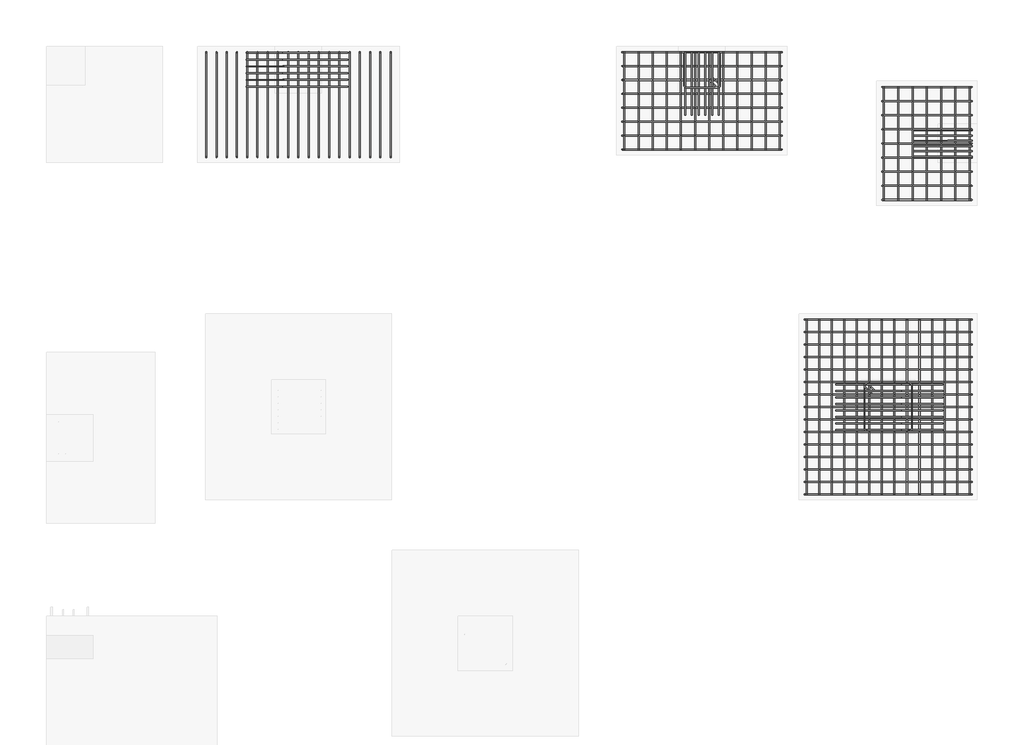
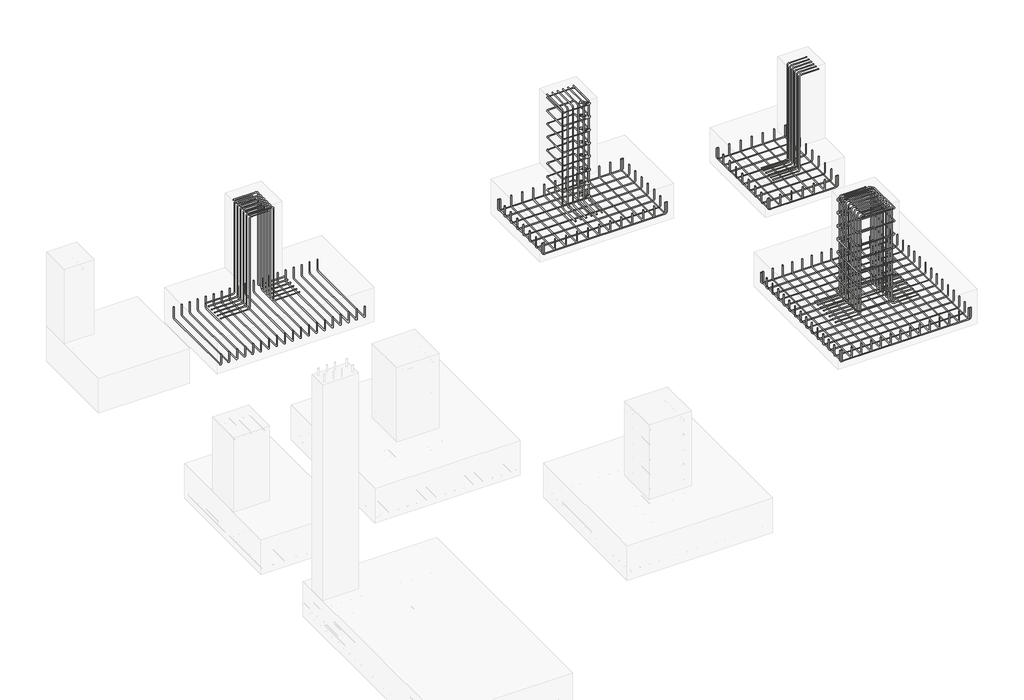
# One storey, part 6 of 6: 15 reinforcing bars.
"""IFC4 building model written with IfcOpenShell, lengths in millimetres."""

from ifc_helpers import new_model, si_unit, point, frame, origin, place, context, project, spatial, polyline, circle_curve, trimmed, segment, composite_curve, source, transform, mapped, element, save
from ifc_brep_helpers import swept_disk

model = new_model("IFC4")

# Units and contexts
model_context = context("Model", 3, world=origin())
ifc_project = project(units=[si_unit("LENGTHUNIT", "METRE", prefix="MILLI")], contexts=[model_context])

# Site, building, storey
site = spatial("IfcSite", under=ifc_project)
building = spatial("IfcBuilding", under=site)
storey = spatial("IfcBuildingStorey", under=building, Elevation=0.0)

# Reinforcing bars
placement = place(None, origin())
reinforcing_bar_shape = source(origin(), model_context, "Body", "SolidModel", [
    swept_disk(composite_curve([segment(polyline([(158482.8232069, -91986.6007776, -254.8), (158482.8232069, -91986.6007776, -377.2)]), True, "CONTINUOUS"), segment(trimmed(circle_curve(frame((158507.8232069, -91986.6007776, -377.2), z_axis=(0.0, -1.0, 0.0), x_axis=(-25.0, 0.0, 0.0)), 25.0), [point((158482.8232069, -91986.6007776, -377.2))], [point((158507.8232069, -91986.6007776, -402.2))], True, "CARTESIAN"), True, "CONTINUOUS"), segment(polyline([(158507.8232069, -91986.6007776, -402.2), (159338.4232069, -91986.6007776, -402.2)]), True, "CONTINUOUS"), segment(trimmed(circle_curve(frame((159338.4232069, -91986.6007776, -377.2), z_axis=(0.0, -1.0, 0.0), x_axis=(0.0, 0.0, -25.0)), 25.0), [point((159338.4232069, -91986.6007776, -402.2))], [point((159363.4232069, -91986.6007776, -377.2))], True, "CARTESIAN"), True, "CONTINUOUS"), segment(polyline([(159363.4232069, -91986.6007776, -377.2), (159363.4232069, -91986.6007776, -254.8)]), True, "CONTINUOUS")], self_intersect=False), 5.0),
])
element("IfcReinforcingBar", 1, at=placement, inside=storey, context=model_context, shape_type="MappedRepresentation", body=[
    mapped(reinforcing_bar_shape, transform((0.0, 0.0, 0.0), x_axis=(1.0, 0.0, 0.0), y_axis=(0.0, 1.0, 0.0), z_axis=(0.0, 0.0, 1.0))),
    mapped(reinforcing_bar_shape, transform((0.0, -138.65, 0.0), x_axis=(1.0, 0.0, 0.0), y_axis=(0.0, 1.0, 0.0), z_axis=(0.0, 0.0, 1.0))),
    mapped(reinforcing_bar_shape, transform((0.0, -277.3, 0.0), x_axis=(1.0, 0.0, 0.0), y_axis=(0.0, 1.0, 0.0), z_axis=(0.0, 0.0, 1.0))),
    mapped(reinforcing_bar_shape, transform((0.0, -415.95, 0.0), x_axis=(1.0, 0.0, 0.0), y_axis=(0.0, 1.0, 0.0), z_axis=(0.0, 0.0, 1.0))),
    mapped(reinforcing_bar_shape, transform((0.0, -554.6, 0.0), x_axis=(1.0, 0.0, 0.0), y_axis=(0.0, 1.0, 0.0), z_axis=(0.0, 0.0, 1.0))),
    mapped(reinforcing_bar_shape, transform((0.0, -693.25, 0.0), x_axis=(1.0, 0.0, 0.0), y_axis=(0.0, 1.0, 0.0), z_axis=(0.0, 0.0, 1.0))),
    mapped(reinforcing_bar_shape, transform((0.0, -831.9, 0.0), x_axis=(1.0, 0.0, 0.0), y_axis=(0.0, 1.0, 0.0), z_axis=(0.0, 0.0, 1.0))),
    mapped(reinforcing_bar_shape, transform((0.0, -970.55, 0.0), x_axis=(1.0, 0.0, 0.0), y_axis=(0.0, 1.0, 0.0), z_axis=(0.0, 0.0, 1.0))),
    mapped(reinforcing_bar_shape, transform((0.0, -1109.2, 0.0), x_axis=(1.0, 0.0, 0.0), y_axis=(0.0, 1.0, 0.0), z_axis=(0.0, 0.0, 1.0))),
])
reinforcing_bar_2_shape = source(origin(), model_context, "Body", "SolidModel", [
    swept_disk(composite_curve([segment(polyline([(158499.498189, -93095.8007776, -254.8), (158499.498189, -93095.8007776, -377.2)]), True, "CONTINUOUS"), segment(trimmed(circle_curve(frame((158499.498189, -93070.8007776, -377.2), z_axis=(1.0, 0.0, 0.0), x_axis=(0.0, -25.0, 0.0)), 25.0), [point((158499.498189, -93095.8007776, -377.2))], [point((158499.498189, -93070.8007776, -402.2))], True, "CARTESIAN"), True, "CONTINUOUS"), segment(polyline([(158499.498189, -93070.8007776, -402.2), (158499.498189, -92011.6007776, -402.2)]), True, "CONTINUOUS"), segment(trimmed(circle_curve(frame((158499.498189, -92011.6007776, -377.2), z_axis=(1.0, 0.0, 0.0), x_axis=(0.0, 0.0, -25.0)), 25.0), [point((158499.498189, -92011.6007776, -402.2))], [point((158499.498189, -91986.6007776, -377.2))], True, "CARTESIAN"), True, "CONTINUOUS"), segment(polyline([(158499.498189, -91986.6007776, -377.2), (158499.498189, -91986.6007776, -254.8)]), True, "CONTINUOUS")], self_intersect=False), 5.0),
])
element("IfcReinforcingBar", 2, at=placement, inside=storey, context=model_context, shape_type="MappedRepresentation", body=[
    mapped(reinforcing_bar_2_shape, transform((0.0, 0.0, 0.0), x_axis=(1.0, 0.0, 0.0), y_axis=(0.0, 1.0, 0.0), z_axis=(0.0, 0.0, 1.0))),
    mapped(reinforcing_bar_2_shape, transform((140.5462786, 0.0, 0.0), x_axis=(1.0, 0.0, 0.0), y_axis=(0.0, 1.0, 0.0), z_axis=(0.0, 0.0, 1.0))),
    mapped(reinforcing_bar_2_shape, transform((281.0925572, 0.0, 0.0), x_axis=(1.0, 0.0, 0.0), y_axis=(0.0, 1.0, 0.0), z_axis=(0.0, 0.0, 1.0))),
    mapped(reinforcing_bar_2_shape, transform((421.6388358, 0.0, 0.0), x_axis=(1.0, 0.0, 0.0), y_axis=(0.0, 1.0, 0.0), z_axis=(0.0, 0.0, 1.0))),
    mapped(reinforcing_bar_2_shape, transform((562.1851144, 0.0, 0.0), x_axis=(1.0, 0.0, 0.0), y_axis=(0.0, 1.0, 0.0), z_axis=(0.0, 0.0, 1.0))),
    mapped(reinforcing_bar_2_shape, transform((702.7313931, 0.0, 0.0), x_axis=(1.0, 0.0, 0.0), y_axis=(0.0, 1.0, 0.0), z_axis=(0.0, 0.0, 1.0))),
    mapped(reinforcing_bar_2_shape, transform((843.2776717, 0.0, 0.0), x_axis=(1.0, 0.0, 0.0), y_axis=(0.0, 1.0, 0.0), z_axis=(0.0, 0.0, 1.0))),
])
reinforcing_bar_3_shape = source(origin(), model_context, "Body", "SolidModel", [
    swept_disk(composite_curve([segment(polyline([(155929.6384274, -91643.7007776, -254.8), (155929.6384274, -91643.7007776, -377.2)]), True, "CONTINUOUS"), segment(trimmed(circle_curve(frame((155954.6384274, -91643.7007776, -377.2), z_axis=(0.0, -1.0, 0.0), x_axis=(-25.0, 0.0, 0.0)), 25.0), [point((155929.6384274, -91643.7007776, -377.2))], [point((155954.6384274, -91643.7007776, -402.2))], True, "CARTESIAN"), True, "CONTINUOUS"), segment(polyline([(155954.6384274, -91643.7007776, -402.2), (157471.0384274, -91643.7007776, -402.2)]), True, "CONTINUOUS"), segment(trimmed(circle_curve(frame((157471.0384274, -91643.7007776, -377.2), z_axis=(0.0, -1.0, 0.0), x_axis=(0.0, 0.0, -25.0)), 25.0), [point((157471.0384274, -91643.7007776, -402.2))], [point((157496.0384274, -91643.7007776, -377.2))], True, "CARTESIAN"), True, "CONTINUOUS"), segment(polyline([(157496.0384274, -91643.7007776, -377.2), (157496.0384274, -91643.7007776, -254.8)]), True, "CONTINUOUS")], self_intersect=False), 5.0),
])
element("IfcReinforcingBar", 3, at=placement, inside=storey, context=model_context, shape_type="MappedRepresentation", body=[
    mapped(reinforcing_bar_3_shape, transform((0.0, 0.0, 0.0), x_axis=(1.0, 0.0, 0.0), y_axis=(0.0, 1.0, 0.0), z_axis=(0.0, 0.0, 1.0))),
    mapped(reinforcing_bar_3_shape, transform((0.0, -136.6857143, 0.0), x_axis=(1.0, 0.0, 0.0), y_axis=(0.0, 1.0, 0.0), z_axis=(0.0, 0.0, 1.0))),
    mapped(reinforcing_bar_3_shape, transform((0.0, -273.3714286, 0.0), x_axis=(1.0, 0.0, 0.0), y_axis=(0.0, 1.0, 0.0), z_axis=(0.0, 0.0, 1.0))),
    mapped(reinforcing_bar_3_shape, transform((0.0, -410.0571429, 0.0), x_axis=(1.0, 0.0, 0.0), y_axis=(0.0, 1.0, 0.0), z_axis=(0.0, 0.0, 1.0))),
    mapped(reinforcing_bar_3_shape, transform((0.0, -546.7428571, 0.0), x_axis=(1.0, 0.0, 0.0), y_axis=(0.0, 1.0, 0.0), z_axis=(0.0, 0.0, 1.0))),
    mapped(reinforcing_bar_3_shape, transform((0.0, -683.4285714, 0.0), x_axis=(1.0, 0.0, 0.0), y_axis=(0.0, 1.0, 0.0), z_axis=(0.0, 0.0, 1.0))),
    mapped(reinforcing_bar_3_shape, transform((0.0, -820.1142857, 0.0), x_axis=(1.0, 0.0, 0.0), y_axis=(0.0, 1.0, 0.0), z_axis=(0.0, 0.0, 1.0))),
    mapped(reinforcing_bar_3_shape, transform((0.0, -956.8, 0.0), x_axis=(1.0, 0.0, 0.0), y_axis=(0.0, 1.0, 0.0), z_axis=(0.0, 0.0, 1.0))),
])
reinforcing_bar_4_shape = source(origin(), model_context, "Body", "SolidModel", [
    swept_disk(composite_curve([segment(polyline([(155951.0650985, -92600.5007776, -254.8), (155951.0650985, -92600.5007776, -377.2)]), True, "CONTINUOUS"), segment(trimmed(circle_curve(frame((155951.0650985, -92575.5007776, -377.2), z_axis=(1.0, 0.0, 0.0), x_axis=(0.0, -25.0, 0.0)), 25.0), [point((155951.0650985, -92600.5007776, -377.2))], [point((155951.0650985, -92575.5007776, -402.2))], True, "CARTESIAN"), True, "CONTINUOUS"), segment(polyline([(155951.0650985, -92575.5007776, -402.2), (155951.0650985, -91668.7007776, -402.2)]), True, "CONTINUOUS"), segment(trimmed(circle_curve(frame((155951.0650985, -91668.7007776, -377.2), z_axis=(1.0, 0.0, 0.0), x_axis=(0.0, 0.0, -25.0)), 25.0), [point((155951.0650985, -91668.7007776, -402.2))], [point((155951.0650985, -91643.7007776, -377.2))], True, "CARTESIAN"), True, "CONTINUOUS"), segment(polyline([(155951.0650985, -91643.7007776, -377.2), (155951.0650985, -91643.7007776, -254.8)]), True, "CONTINUOUS")], self_intersect=False), 5.0),
])
element("IfcReinforcingBar", 4, at=placement, inside=storey, context=model_context, shape_type="MappedRepresentation", body=[
    mapped(reinforcing_bar_4_shape, transform((0.0, 0.0, 0.0), x_axis=(1.0, 0.0, 0.0), y_axis=(0.0, 1.0, 0.0), z_axis=(0.0, 0.0, 1.0))),
    mapped(reinforcing_bar_4_shape, transform((138.7698059, 0.0, 0.0), x_axis=(1.0, 0.0, 0.0), y_axis=(0.0, 1.0, 0.0), z_axis=(0.0, 0.0, 1.0))),
    mapped(reinforcing_bar_4_shape, transform((277.5396119, 0.0, 0.0), x_axis=(1.0, 0.0, 0.0), y_axis=(0.0, 1.0, 0.0), z_axis=(0.0, 0.0, 1.0))),
    mapped(reinforcing_bar_4_shape, transform((416.3094178, 0.0, 0.0), x_axis=(1.0, 0.0, 0.0), y_axis=(0.0, 1.0, 0.0), z_axis=(0.0, 0.0, 1.0))),
    mapped(reinforcing_bar_4_shape, transform((555.0792237, 0.0, 0.0), x_axis=(1.0, 0.0, 0.0), y_axis=(0.0, 1.0, 0.0), z_axis=(0.0, 0.0, 1.0))),
    mapped(reinforcing_bar_4_shape, transform((693.8490296, 0.0, 0.0), x_axis=(1.0, 0.0, 0.0), y_axis=(0.0, 1.0, 0.0), z_axis=(0.0, 0.0, 1.0))),
    mapped(reinforcing_bar_4_shape, transform((832.6188356, 0.0, 0.0), x_axis=(1.0, 0.0, 0.0), y_axis=(0.0, 1.0, 0.0), z_axis=(0.0, 0.0, 1.0))),
    mapped(reinforcing_bar_4_shape, transform((971.3886415, 0.0, 0.0), x_axis=(1.0, 0.0, 0.0), y_axis=(0.0, 1.0, 0.0), z_axis=(0.0, 0.0, 1.0))),
    mapped(reinforcing_bar_4_shape, transform((1110.1584474, 0.0, 0.0), x_axis=(1.0, 0.0, 0.0), y_axis=(0.0, 1.0, 0.0), z_axis=(0.0, 0.0, 1.0))),
    mapped(reinforcing_bar_4_shape, transform((1248.9282533, 0.0, 0.0), x_axis=(1.0, 0.0, 0.0), y_axis=(0.0, 1.0, 0.0), z_axis=(0.0, 0.0, 1.0))),
    mapped(reinforcing_bar_4_shape, transform((1387.6980593, 0.0, 0.0), x_axis=(1.0, 0.0, 0.0), y_axis=(0.0, 1.0, 0.0), z_axis=(0.0, 0.0, 1.0))),
    mapped(reinforcing_bar_4_shape, transform((1526.4678652, 0.0, 0.0), x_axis=(1.0, 0.0, 0.0), y_axis=(0.0, 1.0, 0.0), z_axis=(0.0, 0.0, 1.0))),
])
reinforcing_bar_5_shape = source(origin(), model_context, "Body", "SolidModel", [
    swept_disk(composite_curve([segment(polyline([(151843.3166878, -92676.7007776, -254.8), (151843.3166878, -92676.7007776, -377.2)]), True, "CONTINUOUS"), segment(trimmed(circle_curve(frame((151843.3166878, -92651.7007776, -377.2), z_axis=(1.0, 0.0, 0.0), x_axis=(0.0, -25.0, 0.0)), 25.0), [point((151843.3166878, -92676.7007776, -377.2))], [point((151843.3166878, -92651.7007776, -402.2))], True, "CARTESIAN"), True, "CONTINUOUS"), segment(polyline([(151843.3166878, -92651.7007776, -402.2), (151843.3166878, -91668.7007776, -402.2)]), True, "CONTINUOUS"), segment(trimmed(circle_curve(frame((151843.3166878, -91668.7007776, -377.2), z_axis=(1.0, 0.0, 0.0), x_axis=(0.0, 0.0, -25.0)), 25.0), [point((151843.3166878, -91668.7007776, -402.2))], [point((151843.3166878, -91643.7007776, -377.2))], True, "CARTESIAN"), True, "CONTINUOUS"), segment(polyline([(151843.3166878, -91643.7007776, -377.2), (151843.3166878, -91643.7007776, -254.8)]), True, "CONTINUOUS")], self_intersect=False), 5.0),
])
element("IfcReinforcingBar", 5, at=placement, inside=storey, context=model_context, shape_type="MappedRepresentation", body=[
    mapped(reinforcing_bar_5_shape, transform((0.0, 0.0, 0.0), x_axis=(1.0, 0.0, 0.0), y_axis=(0.0, 1.0, 0.0), z_axis=(0.0, 0.0, 1.0))),
    mapped(reinforcing_bar_5_shape, transform((100.5744351, 0.0, 0.0), x_axis=(1.0, 0.0, 0.0), y_axis=(0.0, 1.0, 0.0), z_axis=(0.0, 0.0, 1.0))),
    mapped(reinforcing_bar_5_shape, transform((201.1488702, 0.0, 0.0), x_axis=(1.0, 0.0, 0.0), y_axis=(0.0, 1.0, 0.0), z_axis=(0.0, 0.0, 1.0))),
    mapped(reinforcing_bar_5_shape, transform((301.7233053, 0.0, 0.0), x_axis=(1.0, 0.0, 0.0), y_axis=(0.0, 1.0, 0.0), z_axis=(0.0, 0.0, 1.0))),
    mapped(reinforcing_bar_5_shape, transform((402.2977404, 0.0, 0.0), x_axis=(1.0, 0.0, 0.0), y_axis=(0.0, 1.0, 0.0), z_axis=(0.0, 0.0, 1.0))),
    mapped(reinforcing_bar_5_shape, transform((502.8721755, 0.0, 0.0), x_axis=(1.0, 0.0, 0.0), y_axis=(0.0, 1.0, 0.0), z_axis=(0.0, 0.0, 1.0))),
    mapped(reinforcing_bar_5_shape, transform((603.4466106, 0.0, 0.0), x_axis=(1.0, 0.0, 0.0), y_axis=(0.0, 1.0, 0.0), z_axis=(0.0, 0.0, 1.0))),
    mapped(reinforcing_bar_5_shape, transform((704.0210458, 0.0, 0.0), x_axis=(1.0, 0.0, 0.0), y_axis=(0.0, 1.0, 0.0), z_axis=(0.0, 0.0, 1.0))),
    mapped(reinforcing_bar_5_shape, transform((804.5954809, 0.0, 0.0), x_axis=(1.0, 0.0, 0.0), y_axis=(0.0, 1.0, 0.0), z_axis=(0.0, 0.0, 1.0))),
    mapped(reinforcing_bar_5_shape, transform((905.169916, 0.0, 0.0), x_axis=(1.0, 0.0, 0.0), y_axis=(0.0, 1.0, 0.0), z_axis=(0.0, 0.0, 1.0))),
    mapped(reinforcing_bar_5_shape, transform((1005.7443511, 0.0, 0.0), x_axis=(1.0, 0.0, 0.0), y_axis=(0.0, 1.0, 0.0), z_axis=(0.0, 0.0, 1.0))),
    mapped(reinforcing_bar_5_shape, transform((1106.3187862, 0.0, 0.0), x_axis=(1.0, 0.0, 0.0), y_axis=(0.0, 1.0, 0.0), z_axis=(0.0, 0.0, 1.0))),
    mapped(reinforcing_bar_5_shape, transform((1206.8932213, 0.0, 0.0), x_axis=(1.0, 0.0, 0.0), y_axis=(0.0, 1.0, 0.0), z_axis=(0.0, 0.0, 1.0))),
    mapped(reinforcing_bar_5_shape, transform((1307.4676564, 0.0, 0.0), x_axis=(1.0, 0.0, 0.0), y_axis=(0.0, 1.0, 0.0), z_axis=(0.0, 0.0, 1.0))),
    mapped(reinforcing_bar_5_shape, transform((1408.0420915, 0.0, 0.0), x_axis=(1.0, 0.0, 0.0), y_axis=(0.0, 1.0, 0.0), z_axis=(0.0, 0.0, 1.0))),
    mapped(reinforcing_bar_5_shape, transform((1508.6165266, 0.0, 0.0), x_axis=(1.0, 0.0, 0.0), y_axis=(0.0, 1.0, 0.0), z_axis=(0.0, 0.0, 1.0))),
    mapped(reinforcing_bar_5_shape, transform((1609.1909617, 0.0, 0.0), x_axis=(1.0, 0.0, 0.0), y_axis=(0.0, 1.0, 0.0), z_axis=(0.0, 0.0, 1.0))),
    mapped(reinforcing_bar_5_shape, transform((1709.7653968, 0.0, 0.0), x_axis=(1.0, 0.0, 0.0), y_axis=(0.0, 1.0, 0.0), z_axis=(0.0, 0.0, 1.0))),
    mapped(reinforcing_bar_5_shape, transform((1810.3398319, 0.0, 0.0), x_axis=(1.0, 0.0, 0.0), y_axis=(0.0, 1.0, 0.0), z_axis=(0.0, 0.0, 1.0))),
])
reinforcing_bar_6_shape = source(origin(), model_context, "Body", "SolidModel", [
    swept_disk(composite_curve([segment(polyline([(157720.823207, -94272.6007776, -254.8), (157720.823207, -94272.6007776, -377.2)]), True, "CONTINUOUS"), segment(trimmed(circle_curve(frame((157745.823207, -94272.6007776, -377.2), z_axis=(0.0, -1.0, 0.0), x_axis=(-25.0, 0.0, 0.0)), 25.0), [point((157720.823207, -94272.6007776, -377.2))], [point((157745.823207, -94272.6007776, -402.2))], True, "CARTESIAN"), True, "CONTINUOUS"), segment(polyline([(157745.823207, -94272.6007776, -402.2), (159338.423207, -94272.6007776, -402.2)]), True, "CONTINUOUS"), segment(trimmed(circle_curve(frame((159338.423207, -94272.6007776, -377.2), z_axis=(0.0, -1.0, 0.0), x_axis=(0.0, 0.0, -25.0)), 25.0), [point((159338.423207, -94272.6007776, -402.2))], [point((159363.423207, -94272.6007776, -377.2))], True, "CARTESIAN"), True, "CONTINUOUS"), segment(polyline([(159363.423207, -94272.6007776, -377.2), (159363.423207, -94272.6007776, -254.8)]), True, "CONTINUOUS")], self_intersect=False), 5.0),
])
element("IfcReinforcingBar", 6, at=placement, inside=storey, context=model_context, shape_type="MappedRepresentation", body=[
    mapped(reinforcing_bar_6_shape, transform((0.0, 0.0, 0.0), x_axis=(1.0, 0.0, 0.0), y_axis=(0.0, 1.0, 0.0), z_axis=(0.0, 0.0, 1.0))),
    mapped(reinforcing_bar_6_shape, transform((0.0, -122.7714286, 0.0), x_axis=(1.0, 0.0, 0.0), y_axis=(0.0, 1.0, 0.0), z_axis=(0.0, 0.0, 1.0))),
    mapped(reinforcing_bar_6_shape, transform((0.0, -245.5428571, 0.0), x_axis=(1.0, 0.0, 0.0), y_axis=(0.0, 1.0, 0.0), z_axis=(0.0, 0.0, 1.0))),
    mapped(reinforcing_bar_6_shape, transform((0.0, -368.3142857, 0.0), x_axis=(1.0, 0.0, 0.0), y_axis=(0.0, 1.0, 0.0), z_axis=(0.0, 0.0, 1.0))),
    mapped(reinforcing_bar_6_shape, transform((0.0, -491.0857143, 0.0), x_axis=(1.0, 0.0, 0.0), y_axis=(0.0, 1.0, 0.0), z_axis=(0.0, 0.0, 1.0))),
    mapped(reinforcing_bar_6_shape, transform((0.0, -613.8571429, 0.0), x_axis=(1.0, 0.0, 0.0), y_axis=(0.0, 1.0, 0.0), z_axis=(0.0, 0.0, 1.0))),
    mapped(reinforcing_bar_6_shape, transform((0.0, -736.6285714, 0.0), x_axis=(1.0, 0.0, 0.0), y_axis=(0.0, 1.0, 0.0), z_axis=(0.0, 0.0, 1.0))),
    mapped(reinforcing_bar_6_shape, transform((0.0, -859.4, 0.0), x_axis=(1.0, 0.0, 0.0), y_axis=(0.0, 1.0, 0.0), z_axis=(0.0, 0.0, 1.0))),
    mapped(reinforcing_bar_6_shape, transform((0.0, -982.1714286, 0.0), x_axis=(1.0, 0.0, 0.0), y_axis=(0.0, 1.0, 0.0), z_axis=(0.0, 0.0, 1.0))),
    mapped(reinforcing_bar_6_shape, transform((0.0, -1104.9428571, 0.0), x_axis=(1.0, 0.0, 0.0), y_axis=(0.0, 1.0, 0.0), z_axis=(0.0, 0.0, 1.0))),
    mapped(reinforcing_bar_6_shape, transform((0.0, -1227.7142857, 0.0), x_axis=(1.0, 0.0, 0.0), y_axis=(0.0, 1.0, 0.0), z_axis=(0.0, 0.0, 1.0))),
    mapped(reinforcing_bar_6_shape, transform((0.0, -1350.4857143, 0.0), x_axis=(1.0, 0.0, 0.0), y_axis=(0.0, 1.0, 0.0), z_axis=(0.0, 0.0, 1.0))),
    mapped(reinforcing_bar_6_shape, transform((0.0, -1473.2571429, 0.0), x_axis=(1.0, 0.0, 0.0), y_axis=(0.0, 1.0, 0.0), z_axis=(0.0, 0.0, 1.0))),
    mapped(reinforcing_bar_6_shape, transform((0.0, -1596.0285714, 0.0), x_axis=(1.0, 0.0, 0.0), y_axis=(0.0, 1.0, 0.0), z_axis=(0.0, 0.0, 1.0))),
    mapped(reinforcing_bar_6_shape, transform((0.0, -1718.8, 0.0), x_axis=(1.0, 0.0, 0.0), y_axis=(0.0, 1.0, 0.0), z_axis=(0.0, 0.0, 1.0))),
])
reinforcing_bar_7_shape = source(origin(), model_context, "Body", "SolidModel", [
    swept_disk(composite_curve([segment(polyline([(157743.6569426, -95991.4007776, -254.8), (157743.6569426, -95991.4007776, -377.2)]), True, "CONTINUOUS"), segment(trimmed(circle_curve(frame((157743.6569426, -95966.4007776, -377.2), z_axis=(1.0, 0.0, 0.0), x_axis=(0.0, -25.0, 0.0)), 25.0), [point((157743.6569426, -95991.4007776, -377.2))], [point((157743.6569426, -95966.4007776, -402.2))], True, "CARTESIAN"), True, "CONTINUOUS"), segment(polyline([(157743.6569426, -95966.4007776, -402.2), (157743.6569426, -94297.6007776, -402.2)]), True, "CONTINUOUS"), segment(trimmed(circle_curve(frame((157743.6569426, -94297.6007776, -377.2), z_axis=(1.0, 0.0, 0.0), x_axis=(0.0, 0.0, -25.0)), 25.0), [point((157743.6569426, -94297.6007776, -402.2))], [point((157743.6569426, -94272.6007776, -377.2))], True, "CARTESIAN"), True, "CONTINUOUS"), segment(polyline([(157743.6569426, -94272.6007776, -377.2), (157743.6569426, -94272.6007776, -254.8)]), True, "CONTINUOUS")], self_intersect=False), 5.0),
])
element("IfcReinforcingBar", 7, at=placement, inside=storey, context=model_context, shape_type="MappedRepresentation", body=[
    mapped(reinforcing_bar_7_shape, transform((0.0, 0.0, 0.0), x_axis=(1.0, 0.0, 0.0), y_axis=(0.0, 1.0, 0.0), z_axis=(0.0, 0.0, 1.0))),
    mapped(reinforcing_bar_7_shape, transform((122.8370266, 0.0, 0.0), x_axis=(1.0, 0.0, 0.0), y_axis=(0.0, 1.0, 0.0), z_axis=(0.0, 0.0, 1.0))),
    mapped(reinforcing_bar_7_shape, transform((245.6740532, 0.0, 0.0), x_axis=(1.0, 0.0, 0.0), y_axis=(0.0, 1.0, 0.0), z_axis=(0.0, 0.0, 1.0))),
    mapped(reinforcing_bar_7_shape, transform((368.5110799, 0.0, 0.0), x_axis=(1.0, 0.0, 0.0), y_axis=(0.0, 1.0, 0.0), z_axis=(0.0, 0.0, 1.0))),
    mapped(reinforcing_bar_7_shape, transform((491.3481065, 0.0, 0.0), x_axis=(1.0, 0.0, 0.0), y_axis=(0.0, 1.0, 0.0), z_axis=(0.0, 0.0, 1.0))),
    mapped(reinforcing_bar_7_shape, transform((614.1851331, 0.0, 0.0), x_axis=(1.0, 0.0, 0.0), y_axis=(0.0, 1.0, 0.0), z_axis=(0.0, 0.0, 1.0))),
    mapped(reinforcing_bar_7_shape, transform((737.0221597, 0.0, 0.0), x_axis=(1.0, 0.0, 0.0), y_axis=(0.0, 1.0, 0.0), z_axis=(0.0, 0.0, 1.0))),
    mapped(reinforcing_bar_7_shape, transform((859.8591864, 0.0, 0.0), x_axis=(1.0, 0.0, 0.0), y_axis=(0.0, 1.0, 0.0), z_axis=(0.0, 0.0, 1.0))),
    mapped(reinforcing_bar_7_shape, transform((982.696213, 0.0, 0.0), x_axis=(1.0, 0.0, 0.0), y_axis=(0.0, 1.0, 0.0), z_axis=(0.0, 0.0, 1.0))),
    mapped(reinforcing_bar_7_shape, transform((1105.5332396, 0.0, 0.0), x_axis=(1.0, 0.0, 0.0), y_axis=(0.0, 1.0, 0.0), z_axis=(0.0, 0.0, 1.0))),
    mapped(reinforcing_bar_7_shape, transform((1228.3702662, 0.0, 0.0), x_axis=(1.0, 0.0, 0.0), y_axis=(0.0, 1.0, 0.0), z_axis=(0.0, 0.0, 1.0))),
    mapped(reinforcing_bar_7_shape, transform((1351.2072929, 0.0, 0.0), x_axis=(1.0, 0.0, 0.0), y_axis=(0.0, 1.0, 0.0), z_axis=(0.0, 0.0, 1.0))),
    mapped(reinforcing_bar_7_shape, transform((1474.0443195, 0.0, 0.0), x_axis=(1.0, 0.0, 0.0), y_axis=(0.0, 1.0, 0.0), z_axis=(0.0, 0.0, 1.0))),
    mapped(reinforcing_bar_7_shape, transform((1596.8813461, 0.0, 0.0), x_axis=(1.0, 0.0, 0.0), y_axis=(0.0, 1.0, 0.0), z_axis=(0.0, 0.0, 1.0))),
])
reinforcing_bar_8_shape = source(origin(), model_context, "Body", "SolidModel", [
    swept_disk(composite_curve([segment(polyline([(159366.2937944, -92412.7007776, 904.5892681), (159144.9937944, -92412.7007776, 904.5892681)]), True, "CONTINUOUS"), segment(trimmed(circle_curve(frame((159144.9937944, -92412.7007776, 884.5892681), z_axis=(0.0, -1.0, 0.0), x_axis=(0.0, 0.0, 20.0)), 20.0), [point((159144.9937944, -92412.7007776, 904.5892681))], [point((159124.9937944, -92412.7007776, 884.5892681))], True, "CARTESIAN"), True, "CONTINUOUS"), segment(polyline([(159124.9937944, -92412.7007776, 884.5892681), (159124.9937944, -92412.7007776, -351.1655515)]), True, "CONTINUOUS"), segment(trimmed(circle_curve(frame((159104.9937944, -92412.7007776, -351.1655515), z_axis=(0.0, 1.0, 0.0), x_axis=(20.0, 0.0, 0.0)), 20.0), [point((159124.9937944, -92412.7007776, -351.1655515))], [point((159104.9937944, -92412.7007776, -371.1655515))], True, "CARTESIAN"), True, "CONTINUOUS"), segment(polyline([(159104.9937944, -92412.7007776, -371.1655515), (158794.7937944, -92412.7007776, -371.1655515)]), True, "CONTINUOUS")], self_intersect=False), 4.0),
])
element("IfcReinforcingBar", 8, at=placement, inside=storey, context=model_context, shape_type="MappedRepresentation", body=[
    mapped(reinforcing_bar_8_shape, transform((0.0, 0.0, 0.0), x_axis=(1.0, 0.0, 0.0), y_axis=(0.0, 1.0, 0.0), z_axis=(0.0, 0.0, 1.0))),
    mapped(reinforcing_bar_8_shape, transform((0.0, -51.4, 0.0), x_axis=(1.0, 0.0, 0.0), y_axis=(0.0, 1.0, 0.0), z_axis=(0.0, 0.0, 1.0))),
    mapped(reinforcing_bar_8_shape, transform((0.0, -102.8, 0.0), x_axis=(1.0, 0.0, 0.0), y_axis=(0.0, 1.0, 0.0), z_axis=(0.0, 0.0, 1.0))),
    mapped(reinforcing_bar_8_shape, transform((0.0, -154.2, 0.0), x_axis=(1.0, 0.0, 0.0), y_axis=(0.0, 1.0, 0.0), z_axis=(0.0, 0.0, 1.0))),
    mapped(reinforcing_bar_8_shape, transform((0.0, -205.6, 0.0), x_axis=(1.0, 0.0, 0.0), y_axis=(0.0, 1.0, 0.0), z_axis=(0.0, 0.0, 1.0))),
    mapped(reinforcing_bar_8_shape, transform((0.0, -257.0, 0.0), x_axis=(1.0, 0.0, 0.0), y_axis=(0.0, 1.0, 0.0), z_axis=(0.0, 0.0, 1.0))),
])
reinforcing_bar_9_shape = source(origin(), model_context, "Body", "SolidModel", [
    swept_disk(composite_curve([segment(polyline([(156547.2384274, -91638.7007776, 924.1703458), (156547.2384274, -91947.8350963, 924.1703458)]), True, "CONTINUOUS"), segment(trimmed(circle_curve(frame((156547.2384274, -91947.8350963, 899.1703458), z_axis=(1.0, 0.0, 0.0), x_axis=(0.0, 0.0, 25.0)), 25.0), [point((156547.2384274, -91947.8350963, 924.1703458))], [point((156547.2384274, -91972.8350963, 899.1703458))], True, "CARTESIAN"), True, "CONTINUOUS"), segment(polyline([(156547.2384274, -91972.8350963, 899.1703458), (156547.2384274, -91972.8350963, -358.8679053)]), True, "CONTINUOUS"), segment(trimmed(circle_curve(frame((156547.2384274, -91997.8350963, -358.8679053), z_axis=(-1.0, 0.0, 0.0), x_axis=(0.0, 25.0, 0.0)), 25.0), [point((156547.2384274, -91972.8350963, -358.8679053))], [point((156547.2384274, -91997.8350963, -383.8679053))], True, "CARTESIAN"), True, "CONTINUOUS"), segment(polyline([(156547.2384274, -91997.8350963, -383.8679053), (156547.2384274, -92261.0007776, -383.8679053)]), True, "CONTINUOUS")], self_intersect=False), 5.0),
])
element("IfcReinforcingBar", 9, at=placement, inside=storey, context=model_context, shape_type="MappedRepresentation", body=[
    mapped(reinforcing_bar_9_shape, transform((0.0, 0.0, 0.0), x_axis=(1.0, 0.0, 0.0), y_axis=(0.0, 1.0, 0.0), z_axis=(0.0, 0.0, 1.0))),
    mapped(reinforcing_bar_9_shape, transform((66.24, 0.0, 0.0), x_axis=(1.0, 0.0, 0.0), y_axis=(0.0, 1.0, 0.0), z_axis=(0.0, 0.0, 1.0))),
    mapped(reinforcing_bar_9_shape, transform((132.48, 0.0, 0.0), x_axis=(1.0, 0.0, 0.0), y_axis=(0.0, 1.0, 0.0), z_axis=(0.0, 0.0, 1.0))),
    mapped(reinforcing_bar_9_shape, transform((198.72, 0.0, 0.0), x_axis=(1.0, 0.0, 0.0), y_axis=(0.0, 1.0, 0.0), z_axis=(0.0, 0.0, 1.0))),
    mapped(reinforcing_bar_9_shape, transform((264.96, 0.0, 0.0), x_axis=(1.0, 0.0, 0.0), y_axis=(0.0, 1.0, 0.0), z_axis=(0.0, 0.0, 1.0))),
    mapped(reinforcing_bar_9_shape, transform((331.2, 0.0, 0.0), x_axis=(1.0, 0.0, 0.0), y_axis=(0.0, 1.0, 0.0), z_axis=(0.0, 0.0, 1.0))),
])
reinforcing_bar_10_shape = source(origin(), model_context, "Body", "SolidModel", [
    swept_disk(composite_curve([segment(polyline([(156817.233846, -91893.4119249, 894.9581133), (156881.580563, -91957.758642, 894.9581133)]), True, "CONTINUOUS"), segment(trimmed(circle_curve(frame((156867.4384274, -91971.9007776, 894.9581133), z_axis=(0.0, 0.0, -1.0), x_axis=(14.14213560000644, 14.14213560000644, 0.0)), 20.0), [point((156881.580563, -91957.758642, 894.9581133))], [point((156867.4384274, -91991.9007776, 894.9581133))], True, "CARTESIAN"), True, "CONTINUOUS"), segment(polyline([(156867.4384274, -91991.9007776, 894.9581133), (156558.2384274, -91991.9007776, 894.9581133)]), True, "CONTINUOUS"), segment(trimmed(circle_curve(frame((156558.2384274, -91971.9007776, 894.9581133), z_axis=(0.0, 0.0, -1.0), x_axis=(0.0, -20.0, 0.0)), 20.0), [point((156558.2384274, -91991.9007776, 894.9581133))], [point((156538.2384274, -91971.9007776, 894.9581133))], True, "CARTESIAN"), True, "CONTINUOUS"), segment(polyline([(156538.2384274, -91971.9007776, 894.9581133), (156538.2384274, -91662.7007776, 894.9581133)]), True, "CONTINUOUS"), segment(trimmed(circle_curve(frame((156558.233181, -91662.7007776, 895.4161832), z_axis=(0.022903497834768336, 0.0, -0.9997376804877032), x_axis=(-19.994753599981777, 0.0, -0.4580698999999413)), 20.0), [point((156538.2384274, -91662.7007776, 894.9581133))], [point((156558.233181, -91642.7007776, 895.4161832))], True, "CARTESIAN"), True, "CONTINUOUS"), segment(polyline([(156558.233181, -91642.7007776, 895.4161832), (156867.4436738, -91642.7007776, 902.5000433)]), True, "CONTINUOUS"), segment(trimmed(circle_curve(frame((156867.4436738, -91662.7007776, 902.5000433), z_axis=(0.022903497834768336, 0.0, -0.9997376804877032), x_axis=(0.0, 20.0, 0.0)), 20.0), [point((156867.4436738, -91642.7007776, 902.5000433))], [point((156887.4384274, -91662.7007776, 902.9581133))], True, "CARTESIAN"), True, "CONTINUOUS"), segment(polyline([(156887.4384274, -91662.7007776, 902.9581133), (156887.4384274, -91971.9007776, 902.9581133)]), True, "CONTINUOUS"), segment(trimmed(circle_curve(frame((156867.4384274, -91971.9007776, 902.9581133), z_axis=(0.0, 0.0, -1.0), x_axis=(20.0, 0.0, 0.0)), 20.0), [point((156887.4384274, -91971.9007776, 902.9581133))], [point((156853.2962918, -91986.0429132, 902.9581133))], True, "CARTESIAN"), True, "CONTINUOUS"), segment(polyline([(156853.2962918, -91986.0429132, 902.9581133), (156788.9495747, -91921.6961961, 902.9581133)]), True, "CONTINUOUS")], self_intersect=False), 4.0),
])
element("IfcReinforcingBar", 10, at=placement, inside=storey, context=model_context, shape_type="MappedRepresentation", body=[
    mapped(reinforcing_bar_10_shape, transform((0.0, 0.0, 0.0), x_axis=(1.0, 0.0, 0.0), y_axis=(0.0, 1.0, 0.0), z_axis=(0.0, 0.0, 1.0))),
    mapped(reinforcing_bar_10_shape, transform((0.0, 0.0, -175.8174244), x_axis=(1.0, 0.0, 0.0), y_axis=(0.0, 1.0, 0.0), z_axis=(0.0, 0.0, 1.0))),
    mapped(reinforcing_bar_10_shape, transform((0.0, 0.0, -351.6348487), x_axis=(1.0, 0.0, 0.0), y_axis=(0.0, 1.0, 0.0), z_axis=(0.0, 0.0, 1.0))),
    mapped(reinforcing_bar_10_shape, transform((0.0, 0.0, -527.4522731), x_axis=(1.0, 0.0, 0.0), y_axis=(0.0, 1.0, 0.0), z_axis=(0.0, 0.0, 1.0))),
    mapped(reinforcing_bar_10_shape, transform((0.0, 0.0, -703.2696975), x_axis=(1.0, 0.0, 0.0), y_axis=(0.0, 1.0, 0.0), z_axis=(0.0, 0.0, 1.0))),
    mapped(reinforcing_bar_10_shape, transform((0.0, 0.0, -879.0871218), x_axis=(1.0, 0.0, 0.0), y_axis=(0.0, 1.0, 0.0), z_axis=(0.0, 0.0, 1.0))),
    mapped(reinforcing_bar_10_shape, transform((0.0, 0.0, -1054.9045462), x_axis=(1.0, 0.0, 0.0), y_axis=(0.0, 1.0, 0.0), z_axis=(0.0, 0.0, 1.0))),
    mapped(reinforcing_bar_10_shape, transform((0.0, 0.0, -1230.7219706), x_axis=(1.0, 0.0, 0.0), y_axis=(0.0, 1.0, 0.0), z_axis=(0.0, 0.0, 1.0))),
])
reinforcing_bar_11_shape = source(origin(), model_context, "Body", "SolidModel", [
    swept_disk(composite_curve([segment(polyline([(152592.4441938, -91982.9007776, 915.2788628), (152878.3232069, -91982.9007776, 915.2788628)]), True, "CONTINUOUS"), segment(trimmed(circle_curve(frame((152878.3232069, -91982.9007776, 890.2788628), z_axis=(0.0, 1.0, 0.0), x_axis=(0.0, 0.0, 25.0)), 25.0), [point((152878.3232069, -91982.9007776, 915.2788628))], [point((152903.3232069, -91982.9007776, 890.2788628))], True, "CARTESIAN"), True, "CONTINUOUS"), segment(polyline([(152903.3232069, -91982.9007776, 890.2788628), (152903.3232069, -91982.9007776, -308.9187146)]), True, "CONTINUOUS"), segment(trimmed(circle_curve(frame((152928.3232069, -91982.9007776, -308.9187146), z_axis=(0.0, -1.0, 0.0), x_axis=(-25.0, 0.0, 0.0)), 25.0), [point((152903.3232069, -91982.9007776, -308.9187146))], [point((152928.3232069, -91982.9007776, -333.9187146))], True, "CARTESIAN"), True, "CONTINUOUS"), segment(polyline([(152928.3232069, -91982.9007776, -333.9187146), (153233.5232069, -91982.9007776, -333.9187146)]), True, "CONTINUOUS")], self_intersect=False), 5.0),
])
element("IfcReinforcingBar", 11, at=placement, inside=storey, context=model_context, shape_type="MappedRepresentation", body=[
    mapped(reinforcing_bar_11_shape, transform((0.0, 0.0, 0.0), x_axis=(1.0, 0.0, 0.0), y_axis=(0.0, 1.0, 0.0), z_axis=(0.0, 0.0, 1.0))),
    mapped(reinforcing_bar_11_shape, transform((0.0, 66.24, 0.0), x_axis=(1.0, 0.0, 0.0), y_axis=(0.0, 1.0, 0.0), z_axis=(0.0, 0.0, 1.0))),
    mapped(reinforcing_bar_11_shape, transform((0.0, 132.48, 0.0), x_axis=(1.0, 0.0, 0.0), y_axis=(0.0, 1.0, 0.0), z_axis=(0.0, 0.0, 1.0))),
    mapped(reinforcing_bar_11_shape, transform((0.0, 198.72, 0.0), x_axis=(1.0, 0.0, 0.0), y_axis=(0.0, 1.0, 0.0), z_axis=(0.0, 0.0, 1.0))),
    mapped(reinforcing_bar_11_shape, transform((0.0, 264.96, 0.0), x_axis=(1.0, 0.0, 0.0), y_axis=(0.0, 1.0, 0.0), z_axis=(0.0, 0.0, 1.0))),
    mapped(reinforcing_bar_11_shape, transform((0.0, 331.2, 0.0), x_axis=(1.0, 0.0, 0.0), y_axis=(0.0, 1.0, 0.0), z_axis=(0.0, 0.0, 1.0))),
])
reinforcing_bar_12_shape = source(origin(), model_context, "Body", "SolidModel", [
    swept_disk(composite_curve([segment(polyline([(152831.513009, -91650.7007776, 884.9542292), (152622.913009, -91650.7007776, 884.9542292)]), True, "CONTINUOUS"), segment(trimmed(circle_curve(frame((152622.913009, -91650.7007776, 864.9542292), z_axis=(0.0, -1.0, 0.0), x_axis=(0.0, 0.0, 20.0)), 20.0), [point((152622.913009, -91650.7007776, 884.9542292))], [point((152602.913009, -91650.7007776, 864.9542292))], True, "CARTESIAN"), True, "CONTINUOUS"), segment(polyline([(152602.913009, -91650.7007776, 864.9542292), (152602.913009, -91650.7007776, -316.9849855)]), True, "CONTINUOUS"), segment(trimmed(circle_curve(frame((152582.913009, -91650.7007776, -316.9849855), z_axis=(0.0, 1.0, 0.0), x_axis=(20.0, 0.0, 0.0)), 20.0), [point((152602.913009, -91650.7007776, -316.9849855))], [point((152582.913009, -91650.7007776, -336.9849855))], True, "CARTESIAN"), True, "CONTINUOUS"), segment(polyline([(152582.913009, -91650.7007776, -336.9849855), (152237.153009, -91650.7007776, -336.9849855)]), True, "CONTINUOUS")], self_intersect=False), 4.0),
])
element("IfcReinforcingBar", 12, at=placement, inside=storey, context=model_context, shape_type="MappedRepresentation", body=[
    mapped(reinforcing_bar_12_shape, transform((0.0, 0.0, 0.0), x_axis=(1.0, 0.0, 0.0), y_axis=(0.0, 1.0, 0.0), z_axis=(0.0, 0.0, 1.0))),
    mapped(reinforcing_bar_12_shape, transform((0.0, -66.64, 0.0), x_axis=(1.0, 0.0, 0.0), y_axis=(0.0, 1.0, 0.0), z_axis=(0.0, 0.0, 1.0))),
    mapped(reinforcing_bar_12_shape, transform((0.0, -133.28, 0.0), x_axis=(1.0, 0.0, 0.0), y_axis=(0.0, 1.0, 0.0), z_axis=(0.0, 0.0, 1.0))),
    mapped(reinforcing_bar_12_shape, transform((0.0, -199.92, 0.0), x_axis=(1.0, 0.0, 0.0), y_axis=(0.0, 1.0, 0.0), z_axis=(0.0, 0.0, 1.0))),
    mapped(reinforcing_bar_12_shape, transform((0.0, -266.56, 0.0), x_axis=(1.0, 0.0, 0.0), y_axis=(0.0, 1.0, 0.0), z_axis=(0.0, 0.0, 1.0))),
    mapped(reinforcing_bar_12_shape, transform((0.0, -333.2, 0.0), x_axis=(1.0, 0.0, 0.0), y_axis=(0.0, 1.0, 0.0), z_axis=(0.0, 0.0, 1.0))),
])
reinforcing_bar_13_shape = source(origin(), model_context, "Body", "SolidModel", [
    swept_disk(composite_curve([segment(polyline([(158669.5918058, -94908.3007776, 933.0070241), (158366.598207, -94908.3007776, 933.0070241)]), True, "CONTINUOUS"), segment(trimmed(circle_curve(frame((158366.598207, -94908.3007776, 908.0070241), z_axis=(0.0, -1.0, 0.0), x_axis=(0.0, 0.0, 25.0)), 25.0), [point((158366.598207, -94908.3007776, 933.0070241))], [point((158341.598207, -94908.3007776, 908.0070241))], True, "CARTESIAN"), True, "CONTINUOUS"), segment(polyline([(158341.598207, -94908.3007776, 908.0070241), (158341.598207, -94908.3007776, -343.6790158)]), True, "CONTINUOUS"), segment(trimmed(circle_curve(frame((158316.598207, -94908.3007776, -343.6790158), z_axis=(0.0, 1.0, 0.0), x_axis=(25.0, 0.0, 0.0)), 25.0), [point((158341.598207, -94908.3007776, -343.6790158))], [point((158316.598207, -94908.3007776, -368.6790158))], True, "CARTESIAN"), True, "CONTINUOUS"), segment(polyline([(158316.598207, -94908.3007776, -368.6790158), (158027.6032021, -94908.3007776, -368.6790158)]), True, "CONTINUOUS")], self_intersect=False), 5.0),
])
element("IfcReinforcingBar", 13, at=placement, inside=storey, context=model_context, shape_type="MappedRepresentation", body=[
    mapped(reinforcing_bar_13_shape, transform((0.0, 0.0, 0.0), x_axis=(1.0, 0.0, 0.0), y_axis=(0.0, 1.0, 0.0), z_axis=(0.0, 0.0, 1.0))),
    mapped(reinforcing_bar_13_shape, transform((0.0, -63.9142857, 0.0), x_axis=(1.0, 0.0, 0.0), y_axis=(0.0, 1.0, 0.0), z_axis=(0.0, 0.0, 1.0))),
    mapped(reinforcing_bar_13_shape, transform((0.0, -127.8285714, 0.0), x_axis=(1.0, 0.0, 0.0), y_axis=(0.0, 1.0, 0.0), z_axis=(0.0, 0.0, 1.0))),
    mapped(reinforcing_bar_13_shape, transform((0.0, -191.7428571, 0.0), x_axis=(1.0, 0.0, 0.0), y_axis=(0.0, 1.0, 0.0), z_axis=(0.0, 0.0, 1.0))),
    mapped(reinforcing_bar_13_shape, transform((0.0, -255.6571429, 0.0), x_axis=(1.0, 0.0, 0.0), y_axis=(0.0, 1.0, 0.0), z_axis=(0.0, 0.0, 1.0))),
    mapped(reinforcing_bar_13_shape, transform((0.0, -319.5714286, 0.0), x_axis=(1.0, 0.0, 0.0), y_axis=(0.0, 1.0, 0.0), z_axis=(0.0, 0.0, 1.0))),
    mapped(reinforcing_bar_13_shape, transform((0.0, -383.4857143, 0.0), x_axis=(1.0, 0.0, 0.0), y_axis=(0.0, 1.0, 0.0), z_axis=(0.0, 0.0, 1.0))),
    mapped(reinforcing_bar_13_shape, transform((0.0, -447.4, 0.0), x_axis=(1.0, 0.0, 0.0), y_axis=(0.0, 1.0, 0.0), z_axis=(0.0, 0.0, 1.0))),
])
reinforcing_bar_14_shape = source(origin(), model_context, "Body", "SolidModel", [
    swept_disk(composite_curve([segment(polyline([(158398.9555958, -95355.7007776, 915.0304286), (158714.473207, -95355.7007776, 915.0304286)]), True, "CONTINUOUS"), segment(trimmed(circle_curve(frame((158714.473207, -95355.7007776, 890.0304286), z_axis=(0.0, 1.0, 0.0), x_axis=(0.0, 0.0, 25.0)), 25.0), [point((158714.473207, -95355.7007776, 915.0304286))], [point((158739.473207, -95355.7007776, 890.0304286))], True, "CARTESIAN"), True, "CONTINUOUS"), segment(polyline([(158739.473207, -95355.7007776, 890.0304286), (158739.473207, -95355.7007776, -342.7230591)]), True, "CONTINUOUS"), segment(trimmed(circle_curve(frame((158764.473207, -95355.7007776, -342.7230591), z_axis=(0.0, -1.0, 0.0), x_axis=(-25.0, 0.0, 0.0)), 25.0), [point((158739.473207, -95355.7007776, -342.7230591))], [point((158764.473207, -95355.7007776, -367.7230591))], True, "CARTESIAN"), True, "CONTINUOUS"), segment(polyline([(158764.473207, -95355.7007776, -367.7230591), (159077.3601497, -95355.7007776, -367.7230591)]), True, "CONTINUOUS")], self_intersect=False), 5.0),
])
element("IfcReinforcingBar", 14, at=placement, inside=storey, context=model_context, shape_type="MappedRepresentation", body=[
    mapped(reinforcing_bar_14_shape, transform((0.0, 0.0, 0.0), x_axis=(1.0, 0.0, 0.0), y_axis=(0.0, 1.0, 0.0), z_axis=(0.0, 0.0, 1.0))),
    mapped(reinforcing_bar_14_shape, transform((0.0, 63.9142857, 0.0), x_axis=(1.0, 0.0, 0.0), y_axis=(0.0, 1.0, 0.0), z_axis=(0.0, 0.0, 1.0))),
    mapped(reinforcing_bar_14_shape, transform((0.0, 127.8285714, 0.0), x_axis=(1.0, 0.0, 0.0), y_axis=(0.0, 1.0, 0.0), z_axis=(0.0, 0.0, 1.0))),
    mapped(reinforcing_bar_14_shape, transform((0.0, 191.7428571, 0.0), x_axis=(1.0, 0.0, 0.0), y_axis=(0.0, 1.0, 0.0), z_axis=(0.0, 0.0, 1.0))),
    mapped(reinforcing_bar_14_shape, transform((0.0, 255.6571429, 0.0), x_axis=(1.0, 0.0, 0.0), y_axis=(0.0, 1.0, 0.0), z_axis=(0.0, 0.0, 1.0))),
    mapped(reinforcing_bar_14_shape, transform((0.0, 319.5714286, 0.0), x_axis=(1.0, 0.0, 0.0), y_axis=(0.0, 1.0, 0.0), z_axis=(0.0, 0.0, 1.0))),
    mapped(reinforcing_bar_14_shape, transform((0.0, 383.4857143, 0.0), x_axis=(1.0, 0.0, 0.0), y_axis=(0.0, 1.0, 0.0), z_axis=(0.0, 0.0, 1.0))),
    mapped(reinforcing_bar_14_shape, transform((0.0, 447.4, 0.0), x_axis=(1.0, 0.0, 0.0), y_axis=(0.0, 1.0, 0.0), z_axis=(0.0, 0.0, 1.0))),
])
reinforcing_bar_15_shape = source(origin(), model_context, "Body", "SolidModel", [
    swept_disk(composite_curve([segment(polyline([(158407.9120597, -94969.5053591, -326.840765), (158343.5653426, -94905.158642, -326.840765)]), True, "CONTINUOUS"), segment(trimmed(circle_curve(frame((158329.423207, -94919.3007776, -326.840765), z_axis=(0.0, 0.0, 1.0), x_axis=(14.142135599977337, 14.14213560000644, 0.0)), 20.0), [point((158343.5653426, -94905.158642, -326.840765))], [point((158309.423207, -94919.3007776, -326.840765))], True, "CARTESIAN"), True, "CONTINUOUS"), segment(polyline([(158309.423207, -94919.3007776, -326.840765), (158309.423207, -95344.7007776, -326.840765)]), True, "CONTINUOUS"), segment(trimmed(circle_curve(frame((158329.423207, -95344.7007776, -326.840765), z_axis=(0.0, 0.0, 1.0), x_axis=(-20.0, 0.0, 0.0)), 20.0), [point((158309.423207, -95344.7007776, -326.840765))], [point((158329.423207, -95364.7007776, -326.840765))], True, "CARTESIAN"), True, "CONTINUOUS"), segment(polyline([(158329.423207, -95364.7007776, -326.840765), (158754.823207, -95364.7007776, -326.840765)]), True, "CONTINUOUS"), segment(trimmed(circle_curve(frame((158754.823207, -95344.7037317, -327.1845045), z_axis=(0.0, 0.017186975385128117, 0.999852293029881), x_axis=(0.0, -19.997045899988734, 0.3437395000000265)), 20.0), [point((158754.823207, -95364.7007776, -326.840765))], [point((158774.823207, -95344.7037317, -327.1845045))], True, "CARTESIAN"), True, "CONTINUOUS"), segment(polyline([(158774.823207, -95344.7037317, -327.1845045), (158774.823207, -94919.2978235, -334.4970255)]), True, "CONTINUOUS"), segment(trimmed(circle_curve(frame((158754.823207, -94919.2978235, -334.4970255), z_axis=(0.0, 0.017186975385128117, 0.999852293029881), x_axis=(20.0, 0.0, 0.0)), 20.0), [point((158774.823207, -94919.2978235, -334.4970255))], [point((158754.823207, -94899.3007776, -334.840765))], True, "CARTESIAN"), True, "CONTINUOUS"), segment(polyline([(158754.823207, -94899.3007776, -334.840765), (158329.423207, -94899.3007776, -334.840765)]), True, "CONTINUOUS"), segment(trimmed(circle_curve(frame((158329.423207, -94919.3007776, -334.840765), z_axis=(0.0, 0.0, 1.0), x_axis=(0.0, 20.0, 0.0)), 20.0), [point((158329.423207, -94899.3007776, -334.840765))], [point((158315.2810714, -94933.4429132, -334.840765))], True, "CARTESIAN"), True, "CONTINUOUS"), segment(polyline([(158315.2810714, -94933.4429132, -334.840765), (158379.6277885, -94997.7896303, -334.840765)]), True, "CONTINUOUS")], self_intersect=False), 4.0),
])
element("IfcReinforcingBar", 15, at=placement, inside=storey, context=model_context, shape_type="MappedRepresentation", body=[
    mapped(reinforcing_bar_15_shape, transform((0.0, 0.0, 0.0), x_axis=(1.0, 0.0, 0.0), y_axis=(0.0, 1.0, 0.0), z_axis=(0.0, 0.0, 1.0))),
    mapped(reinforcing_bar_15_shape, transform((0.0, 0.0, 174.4633022), x_axis=(1.0, 0.0, 0.0), y_axis=(0.0, 1.0, 0.0), z_axis=(0.0, 0.0, 1.0))),
    mapped(reinforcing_bar_15_shape, transform((0.0, 0.0, 348.9266043), x_axis=(1.0, 0.0, 0.0), y_axis=(0.0, 1.0, 0.0), z_axis=(0.0, 0.0, 1.0))),
    mapped(reinforcing_bar_15_shape, transform((0.0, 0.0, 523.3899065), x_axis=(1.0, 0.0, 0.0), y_axis=(0.0, 1.0, 0.0), z_axis=(0.0, 0.0, 1.0))),
    mapped(reinforcing_bar_15_shape, transform((0.0, 0.0, 697.8532086), x_axis=(1.0, 0.0, 0.0), y_axis=(0.0, 1.0, 0.0), z_axis=(0.0, 0.0, 1.0))),
    mapped(reinforcing_bar_15_shape, transform((0.0, 0.0, 872.3165108), x_axis=(1.0, 0.0, 0.0), y_axis=(0.0, 1.0, 0.0), z_axis=(0.0, 0.0, 1.0))),
    mapped(reinforcing_bar_15_shape, transform((0.0, 0.0, 1046.7798129), x_axis=(1.0, 0.0, 0.0), y_axis=(0.0, 1.0, 0.0), z_axis=(0.0, 0.0, 1.0))),
    mapped(reinforcing_bar_15_shape, transform((0.0, 0.0, 1221.2431151), x_axis=(1.0, 0.0, 0.0), y_axis=(0.0, 1.0, 0.0), z_axis=(0.0, 0.0, 1.0))),
])

save(model, "model.ifc")

# Revit data of these elements
# Elements 1, 2, 3, 4, 5, 6, 7, 8, 9, 10, 11, 12, 13, 14, 15 (IfcReinforcingBar)
#   Phase Created = New Construction
